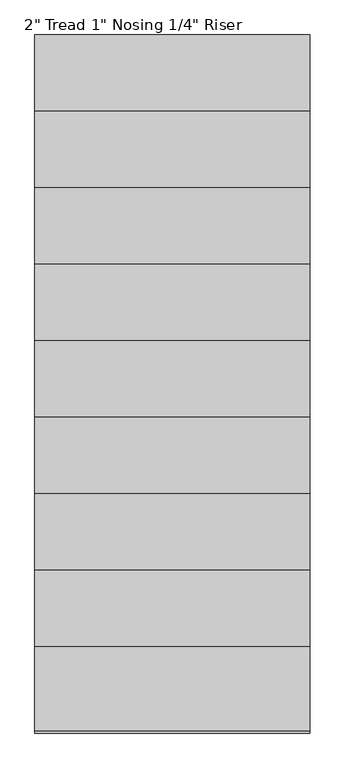
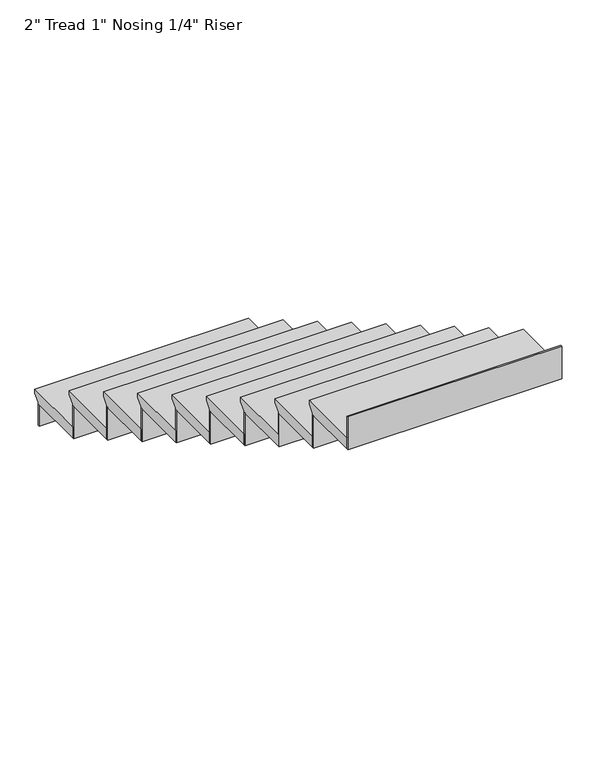
"""IFC4 building model written with IfcOpenShell, lengths in millimetres: stair flight geometry."""

from ifc_helpers import new_model, si_unit, origin, place, context, project, spatial, faceted_brep, source, transform, mapped, element, save


def stair_flight_98d8f9c6(model_context):
    return source(origin(), model_context, "Body", "Brep", [
        faceted_brep([(-4315.1137331, -4241.0593836, 12873.5714861), (-4315.1137331, -4241.0593836, 12892.6214861), (-3400.7137331, -4241.0593836, 12892.6214861), (-3400.7137331, -4241.0593836, 12873.5714861), (-4315.1137331, -4266.4593836, 12848.1714861), (-3400.7137331, -4266.4593836, 12848.1714861), (-4315.1137331, -4520.4593836, 12892.6214861), (-3400.7137331, -4520.4593836, 12892.6214861), (-3400.7137331, -4266.4593836, 12841.8214861), (-3400.7137331, -4520.4593836, 12841.8214861), (-4315.1137331, -4520.4593836, 12841.8214861), (-4315.1137331, -4266.4593836, 12841.8214861)], [[[0, 1, 2, 3]], [[4, 0, 3, 5]], [[2, 1, 6, 7]], [[8, 9, 10, 11]], [[2, 7, 9, 8, 5, 3]], [[8, 11, 4, 5]], [[6, 1, 0, 4, 11, 10]], [[7, 6, 10, 9]]]),
        faceted_brep([(-4315.1137331, -4266.4593836, 12841.8214861), (-4315.1137331, -4266.4593836, 12744.7725604), (-4315.1137331, -4272.8093836, 12744.7725604), (-4315.1137331, -4272.8093836, 12841.8214861), (-3400.7137331, -4266.4593836, 12841.8214861), (-3400.7137331, -4272.8093836, 12841.8214861), (-3400.7137331, -4272.8093836, 12744.7725604), (-3400.7137331, -4266.4593836, 12744.7725604)], [[[0, 1, 2, 3]], [[4, 5, 6, 7]], [[1, 0, 4, 7]], [[2, 1, 7, 6]], [[3, 2, 6, 5]], [[0, 3, 5, 4]]]),
        faceted_brep([(-4315.1137331, -4520.4593836, 12989.6704118), (-4315.1137331, -4520.4593836, 12841.8214861), (-4315.1137331, -4526.8093836, 12841.8214861), (-4315.1137331, -4526.8093836, 12989.6704118), (-3400.7137331, -4520.4593836, 12989.6704118), (-3400.7137331, -4526.8093836, 12989.6704118), (-3400.7137331, -4526.8093836, 12841.8214861), (-3400.7137331, -4520.4593836, 12841.8214861)], [[[0, 1, 2, 3]], [[4, 5, 6, 7]], [[1, 0, 4, 7]], [[2, 1, 7, 6]], [[3, 2, 6, 5]], [[0, 3, 5, 4]]]),
        faceted_brep([(-3400.7137331, -4495.0593836, 13040.4704118), (-4315.1137331, -4495.0593836, 13040.4704118), (-4315.1137331, -4774.4593836, 13040.4704118), (-3400.7137331, -4774.4593836, 13040.4704118), (-3400.7137331, -4520.4593836, 12989.6704118), (-3400.7137331, -4774.4593836, 12989.6704118), (-4315.1137331, -4774.4593836, 12989.6704118), (-4315.1137331, -4520.4593836, 12989.6704118), (-3400.7137331, -4520.4593836, 12996.0204118), (-3400.7137331, -4495.0593836, 13021.4204118), (-4315.1137331, -4520.4593836, 12996.0204118), (-4315.1137331, -4495.0593836, 13021.4204118)], [[[0, 1, 2, 3]], [[4, 5, 6, 7]], [[0, 3, 5, 4, 8, 9]], [[4, 7, 10, 8]], [[2, 1, 11, 10, 7, 6]], [[3, 2, 6, 5]], [[11, 1, 0, 9]], [[10, 11, 9, 8]]]),
        faceted_brep([(-4315.1137331, -4774.4593836, 13137.5193375), (-4315.1137331, -4774.4593836, 12989.6704118), (-4315.1137331, -4780.8093836, 12989.6704118), (-4315.1137331, -4780.8093836, 13137.5193375), (-3400.7137331, -4774.4593836, 13137.5193375), (-3400.7137331, -4780.8093836, 13137.5193375), (-3400.7137331, -4780.8093836, 12989.6704118), (-3400.7137331, -4774.4593836, 12989.6704118)], [[[0, 1, 2, 3]], [[4, 5, 6, 7]], [[1, 0, 4, 7]], [[2, 1, 7, 6]], [[3, 2, 6, 5]], [[0, 3, 5, 4]]]),
        faceted_brep([(-3400.7137331, -4749.0593836, 13188.3193375), (-4315.1137331, -4749.0593836, 13188.3193375), (-4315.1137331, -5028.4593836, 13188.3193375), (-3400.7137331, -5028.4593836, 13188.3193375), (-3400.7137331, -4774.4593836, 13137.5193375), (-3400.7137331, -5028.4593836, 13137.5193375), (-4315.1137331, -5028.4593836, 13137.5193375), (-4315.1137331, -4774.4593836, 13137.5193375), (-3400.7137331, -4774.4593836, 13143.8693375), (-3400.7137331, -4749.0593836, 13169.2693375), (-4315.1137331, -4774.4593836, 13143.8693375), (-4315.1137331, -4749.0593836, 13169.2693375)], [[[0, 1, 2, 3]], [[4, 5, 6, 7]], [[0, 3, 5, 4, 8, 9]], [[4, 7, 10, 8]], [[2, 1, 11, 10, 7, 6]], [[3, 2, 6, 5]], [[11, 1, 0, 9]], [[10, 11, 9, 8]]]),
        faceted_brep([(-4315.1137331, -5028.4593836, 13285.3682632), (-4315.1137331, -5028.4593836, 13137.5193375), (-4315.1137331, -5034.8093836, 13137.5193375), (-4315.1137331, -5034.8093836, 13285.3682632), (-3400.7137331, -5028.4593836, 13285.3682632), (-3400.7137331, -5034.8093836, 13285.3682632), (-3400.7137331, -5034.8093836, 13137.5193375), (-3400.7137331, -5028.4593836, 13137.5193375)], [[[0, 1, 2, 3]], [[4, 5, 6, 7]], [[1, 0, 4, 7]], [[2, 1, 7, 6]], [[3, 2, 6, 5]], [[0, 3, 5, 4]]]),
        faceted_brep([(-3400.7137331, -5003.0593836, 13336.1682632), (-4315.1137331, -5003.0593836, 13336.1682632), (-4315.1137331, -5282.4593836, 13336.1682632), (-3400.7137331, -5282.4593836, 13336.1682632), (-3400.7137331, -5028.4593836, 13285.3682632), (-3400.7137331, -5282.4593836, 13285.3682632), (-4315.1137331, -5282.4593836, 13285.3682632), (-4315.1137331, -5028.4593836, 13285.3682632), (-3400.7137331, -5028.4593836, 13291.7182632), (-3400.7137331, -5003.0593836, 13317.1182632), (-4315.1137331, -5028.4593836, 13291.7182632), (-4315.1137331, -5003.0593836, 13317.1182632)], [[[0, 1, 2, 3]], [[4, 5, 6, 7]], [[0, 3, 5, 4, 8, 9]], [[4, 7, 10, 8]], [[2, 1, 11, 10, 7, 6]], [[3, 2, 6, 5]], [[11, 1, 0, 9]], [[10, 11, 9, 8]]]),
        faceted_brep([(-4315.1137331, -5282.4593836, 13433.2171889), (-4315.1137331, -5282.4593836, 13285.3682632), (-4315.1137331, -5288.8093836, 13285.3682632), (-4315.1137331, -5288.8093836, 13433.2171889), (-3400.7137331, -5282.4593836, 13433.2171889), (-3400.7137331, -5288.8093836, 13433.2171889), (-3400.7137331, -5288.8093836, 13285.3682632), (-3400.7137331, -5282.4593836, 13285.3682632)], [[[0, 1, 2, 3]], [[4, 5, 6, 7]], [[1, 0, 4, 7]], [[2, 1, 7, 6]], [[3, 2, 6, 5]], [[0, 3, 5, 4]]]),
        faceted_brep([(-3400.7137331, -5257.0593836, 13484.0171889), (-4315.1137331, -5257.0593836, 13484.0171889), (-4315.1137331, -5536.4593836, 13484.0171889), (-3400.7137331, -5536.4593836, 13484.0171889), (-3400.7137331, -5282.4593836, 13433.2171889), (-3400.7137331, -5536.4593836, 13433.2171889), (-4315.1137331, -5536.4593836, 13433.2171889), (-4315.1137331, -5282.4593836, 13433.2171889), (-3400.7137331, -5282.4593836, 13439.5671889), (-3400.7137331, -5257.0593836, 13464.9671889), (-4315.1137331, -5282.4593836, 13439.5671889), (-4315.1137331, -5257.0593836, 13464.9671889)], [[[0, 1, 2, 3]], [[4, 5, 6, 7]], [[0, 3, 5, 4, 8, 9]], [[4, 7, 10, 8]], [[2, 1, 11, 10, 7, 6]], [[3, 2, 6, 5]], [[11, 1, 0, 9]], [[10, 11, 9, 8]]]),
        faceted_brep([(-4315.1137331, -5536.4593836, 13581.0661146), (-4315.1137331, -5536.4593836, 13433.2171889), (-4315.1137331, -5542.8093836, 13433.2171889), (-4315.1137331, -5542.8093836, 13581.0661146), (-3400.7137331, -5536.4593836, 13581.0661146), (-3400.7137331, -5542.8093836, 13581.0661146), (-3400.7137331, -5542.8093836, 13433.2171889), (-3400.7137331, -5536.4593836, 13433.2171889)], [[[0, 1, 2, 3]], [[4, 5, 6, 7]], [[1, 0, 4, 7]], [[2, 1, 7, 6]], [[3, 2, 6, 5]], [[0, 3, 5, 4]]]),
        faceted_brep([(-3400.7137331, -5511.0593836, 13631.8661146), (-4315.1137331, -5511.0593836, 13631.8661146), (-4315.1137331, -5790.4593836, 13631.8661146), (-3400.7137331, -5790.4593836, 13631.8661146), (-3400.7137331, -5536.4593836, 13581.0661146), (-3400.7137331, -5790.4593836, 13581.0661146), (-4315.1137331, -5790.4593836, 13581.0661146), (-4315.1137331, -5536.4593836, 13581.0661146), (-3400.7137331, -5536.4593836, 13587.4161146), (-3400.7137331, -5511.0593836, 13612.8161146), (-4315.1137331, -5536.4593836, 13587.4161146), (-4315.1137331, -5511.0593836, 13612.8161146)], [[[0, 1, 2, 3]], [[4, 5, 6, 7]], [[0, 3, 5, 4, 8, 9]], [[4, 7, 10, 8]], [[2, 1, 11, 10, 7, 6]], [[3, 2, 6, 5]], [[11, 1, 0, 9]], [[10, 11, 9, 8]]]),
        faceted_brep([(-4315.1137331, -5790.4593836, 13728.9150403), (-4315.1137331, -5790.4593836, 13581.0661146), (-4315.1137331, -5796.8093836, 13581.0661146), (-4315.1137331, -5796.8093836, 13728.9150403), (-3400.7137331, -5790.4593836, 13728.9150403), (-3400.7137331, -5796.8093836, 13728.9150403), (-3400.7137331, -5796.8093836, 13581.0661146), (-3400.7137331, -5790.4593836, 13581.0661146)], [[[0, 1, 2, 3]], [[4, 5, 6, 7]], [[1, 0, 4, 7]], [[2, 1, 7, 6]], [[3, 2, 6, 5]], [[0, 3, 5, 4]]]),
        faceted_brep([(-3400.7137331, -5765.0593836, 13779.7150403), (-4315.1137331, -5765.0593836, 13779.7150403), (-4315.1137331, -6044.4593836, 13779.7150403), (-3400.7137331, -6044.4593836, 13779.7150403), (-3400.7137331, -5790.4593836, 13728.9150403), (-3400.7137331, -6044.4593836, 13728.9150403), (-4315.1137331, -6044.4593836, 13728.9150403), (-4315.1137331, -5790.4593836, 13728.9150403), (-3400.7137331, -5790.4593836, 13735.2650403), (-3400.7137331, -5765.0593836, 13760.6650403), (-4315.1137331, -5790.4593836, 13735.2650403), (-4315.1137331, -5765.0593836, 13760.6650403)], [[[0, 1, 2, 3]], [[4, 5, 6, 7]], [[0, 3, 5, 4, 8, 9]], [[4, 7, 10, 8]], [[2, 1, 11, 10, 7, 6]], [[3, 2, 6, 5]], [[11, 1, 0, 9]], [[10, 11, 9, 8]]]),
        faceted_brep([(-4315.1137331, -6044.4593836, 13876.763966), (-4315.1137331, -6044.4593836, 13728.9150403), (-4315.1137331, -6050.8093836, 13728.9150403), (-4315.1137331, -6050.8093836, 13876.763966), (-3400.7137331, -6044.4593836, 13876.763966), (-3400.7137331, -6050.8093836, 13876.763966), (-3400.7137331, -6050.8093836, 13728.9150403), (-3400.7137331, -6044.4593836, 13728.9150403)], [[[0, 1, 2, 3]], [[4, 5, 6, 7]], [[1, 0, 4, 7]], [[2, 1, 7, 6]], [[3, 2, 6, 5]], [[0, 3, 5, 4]]]),
        faceted_brep([(-3400.7137331, -6019.0593836, 13927.563966), (-4315.1137331, -6019.0593836, 13927.563966), (-4315.1137331, -6298.4593836, 13927.563966), (-3400.7137331, -6298.4593836, 13927.563966), (-3400.7137331, -6044.4593836, 13876.763966), (-3400.7137331, -6298.4593836, 13876.763966), (-4315.1137331, -6298.4593836, 13876.763966), (-4315.1137331, -6044.4593836, 13876.763966), (-3400.7137331, -6044.4593836, 13883.113966), (-3400.7137331, -6019.0593836, 13908.513966), (-4315.1137331, -6044.4593836, 13883.113966), (-4315.1137331, -6019.0593836, 13908.513966)], [[[0, 1, 2, 3]], [[4, 5, 6, 7]], [[0, 3, 5, 4, 8, 9]], [[4, 7, 10, 8]], [[2, 1, 11, 10, 7, 6]], [[3, 2, 6, 5]], [[11, 1, 0, 9]], [[10, 11, 9, 8]]]),
        faceted_brep([(-4315.1137331, -6552.4593836, 14172.4618174), (-4315.1137331, -6552.4593836, 14024.6128917), (-4315.1137331, -6558.8093836, 14024.6128917), (-4315.1137331, -6558.8093836, 14172.4618174), (-3400.7137331, -6552.4593836, 14172.4618174), (-3400.7137331, -6558.8093836, 14172.4618174), (-3400.7137331, -6558.8093836, 14024.6128917), (-3400.7137331, -6552.4593836, 14024.6128917)], [[[0, 1, 2, 3]], [[4, 5, 6, 7]], [[1, 0, 4, 7]], [[2, 1, 7, 6]], [[3, 2, 6, 5]], [[0, 3, 5, 4]]]),
        faceted_brep([(-4315.1137331, -6298.4593836, 14024.6128917), (-4315.1137331, -6298.4593836, 13876.763966), (-4315.1137331, -6304.8093836, 13876.763966), (-4315.1137331, -6304.8093836, 14024.6128917), (-3400.7137331, -6298.4593836, 14024.6128917), (-3400.7137331, -6304.8093836, 14024.6128917), (-3400.7137331, -6304.8093836, 13876.763966), (-3400.7137331, -6298.4593836, 13876.763966)], [[[0, 1, 2, 3]], [[4, 5, 6, 7]], [[1, 0, 4, 7]], [[2, 1, 7, 6]], [[3, 2, 6, 5]], [[0, 3, 5, 4]]]),
        faceted_brep([(-3400.7137331, -6552.4593836, 14075.4128917), (-3400.7137331, -6527.0593836, 14075.4128917), (-3400.7137331, -6273.0593836, 14075.4128917), (-4315.1137331, -6273.0593836, 14075.4128917), (-4315.1137331, -6552.4593836, 14075.4128917), (-3400.7137331, -6527.0593836, 14024.6128917), (-3400.7137331, -6552.4593836, 14024.6128917), (-4315.1137331, -6552.4593836, 14024.6128917), (-4315.1137331, -6298.4593836, 14024.6128917), (-3400.7137331, -6298.4593836, 14024.6128917), (-3400.7137331, -6298.4593836, 14030.9628917), (-3400.7137331, -6273.0593836, 14056.3628917), (-4315.1137331, -6298.4593836, 14030.9628917), (-4315.1137331, -6273.0593836, 14056.3628917)], [[[0, 1, 2, 3, 4]], [[5, 6, 7, 8, 9]], [[1, 0, 6, 5]], [[2, 1, 5, 9, 10, 11]], [[9, 8, 12, 10]], [[4, 3, 13, 12, 8, 7]], [[0, 4, 7, 6]], [[13, 3, 2, 11]], [[12, 13, 11, 10]]]),
    ])


if __name__ == "__main__":
    model = new_model("IFC4")
    model_context = context("Model", 3, world=origin())
    ifc_project = project(units=[si_unit("LENGTHUNIT", "METRE", prefix="MILLI")], contexts=[model_context])
    site = spatial("IfcSite", under=ifc_project)
    building = spatial("IfcBuilding", under=site)
    placement = place(None, origin())
    stair_flight_shape = stair_flight_98d8f9c6(model_context)
    element("IfcStairFlight", 1, ObjectType="2\" Tread 1\" Nosing 1/4\" Riser", at=placement, inside=building, context=model_context, shape_type="MappedRepresentation", body=[
        mapped(stair_flight_shape, transform((0.0, 0.0, 0.0), x_axis=(1.0, 0.0, 0.0), y_axis=(0.0, 1.0, 0.0), z_axis=(0.0, 0.0, 1.0))),
    ])
    save(model, "model.ifc")
